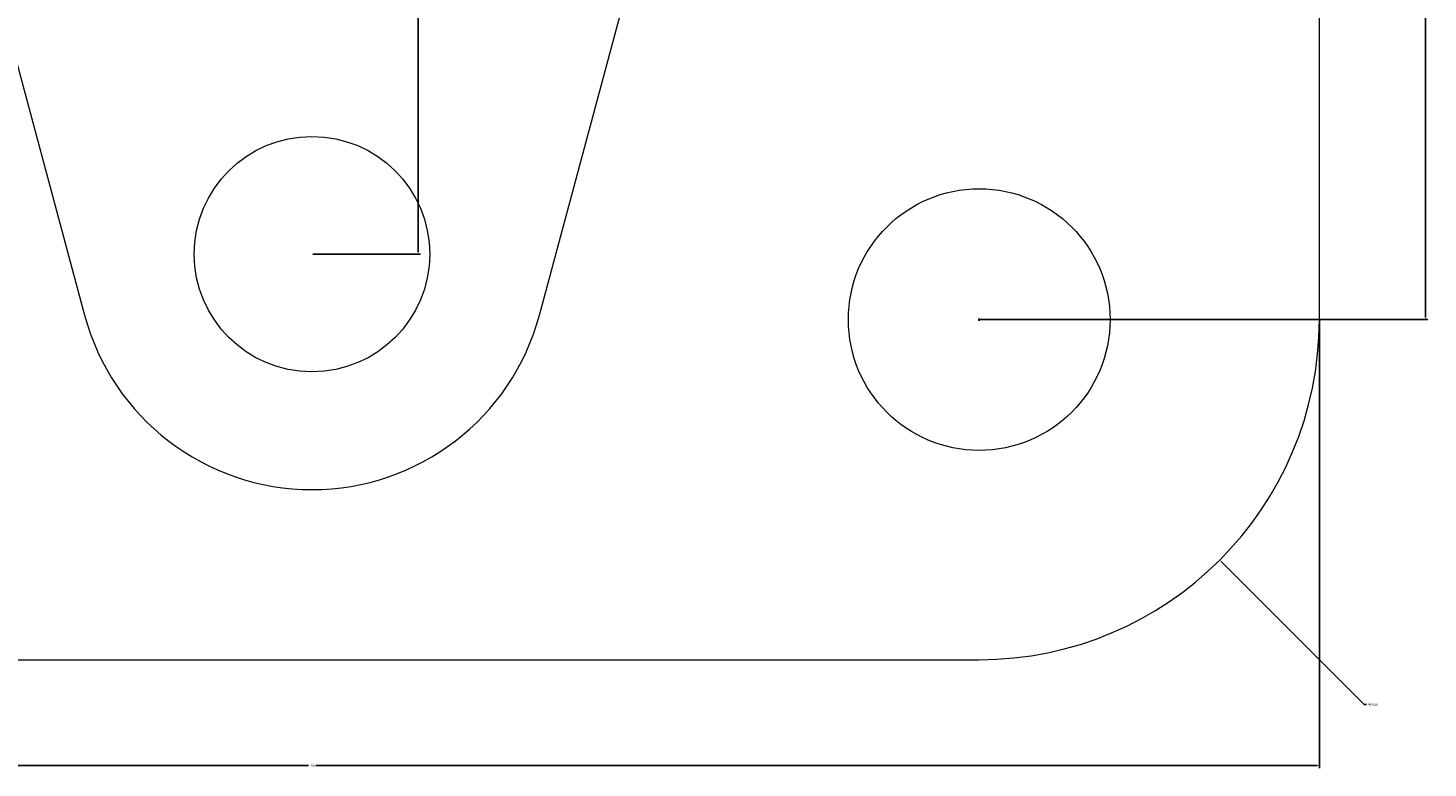
# Model space of a CAD drawing. Units: millimetres. Extents: x 2597 to 2768, y 1809 to 1980.
# Tile 4 of 7: x 2661 to 2768, y 1809 to 1866. Entities that reach past the tile are written whole.
import ezdxf

# ---------------------------------------------------------------- set-up
doc = ezdxf.new("R2010")
doc.units = ezdxf.units.MM
doc.layers.add('M-CONS', color=8, linetype='Continuous', lineweight=18)
doc.layers.add('M-DIMS', color=2, linetype='Continuous', lineweight=18)
doc.styles.get("Standard").update_dxf_attribs({"font": 'arial.ttf'})
doc.dimstyles.get("Standard").update_dxf_attribs({"dimtxt": 0.18, "dimasz": 0.18, "dimexe": 0.18, "dimexo": 0.0625, "dimgap": 0.09, "dimtad": 0, "dimtih": 1, "dimtoh": 1, "dimdec": 4, "dimzin": 0, "dimdsep": 46, "dimtxsty": 'Standard', "dimcen": 0.09, "dimadec": 0, "dimazin": 0, "dimtfac": 1, "dimtdec": 4, "dimtofl": 0, "dimtmove": 0, "dimatfit": 3, "dimfxl": 1, "dimtolj": 1, "dimtzin": 0, "dimarcsym": 0})

# ---------------------------------------------------------------- blocks, each defined once
blk = doc.blocks.new('*D3')
at = {"layer": 'Defpoints', "color": 0, "transparency": 16777216}
for p in [(2605.78, 1843.43), (2759.78, 1843.43), (2759.78, 1809.33)]:
    blk.add_point(p, dxfattribs=at)
at = {"layer": 'M-DIMS', "color": 0, "lineweight": -2, "transparency": 16777216}
for p, q in [((2605.78, 1843.37), (2605.78, 1809.15)), ((2759.78, 1843.37), (2759.78, 1809.15)), ((2605.96, 1809.33), (2682.5, 1809.33)), ((2759.6, 1809.33), (2683.06, 1809.33))]:
    blk.add_line(p, q, dxfattribs=at)
at = {"layer": 'M-DIMS', "color": 0, "transparency": 16777216}
for points in [[(2605.96, 1809.36), (2605.96, 1809.3), (2605.78, 1809.33)], [(2759.6, 1809.36), (2759.6, 1809.3), (2759.78, 1809.33)]]:
    blk.add_solid(points, dxfattribs=at)
at = {"layer": 'M-DIMS', "color": 0, "transparency": 16777216, "insert": (2682.78, 1809.33), "char_height": 0.18, "attachment_point": 5}
blk.add_mtext('\\A1;154', dxfattribs=at)
blk = doc.blocks.new('*D6')
at = {"layer": 'Defpoints', "color": 0, "transparency": 16777216}
for p in [(2733.78, 1945.43), (2767.88, 1945.43), (2733.78, 1843.43)]:
    blk.add_point(p, dxfattribs=at)
at = {"layer": 'M-DIMS', "color": 0, "lineweight": -2, "transparency": 16777216}
for p, q in [((2733.84, 1945.43), (2768.06, 1945.43)), ((2767.88, 1945.25), (2767.88, 1894.61)), ((2767.88, 1843.61), (2767.88, 1894.25)), ((2733.84, 1843.43), (2768.06, 1843.43))]:
    blk.add_line(p, q, dxfattribs=at)
at = {"layer": 'M-DIMS', "color": 0, "transparency": 16777216}
for points in [[(2767.85, 1945.25), (2767.91, 1945.25), (2767.88, 1945.43)], [(2767.85, 1843.61), (2767.91, 1843.61), (2767.88, 1843.43)]]:
    blk.add_solid(points, dxfattribs=at)
at = {"layer": 'M-DIMS', "color": 0, "transparency": 16777216, "insert": (2767.88, 1894.43), "char_height": 0.18, "attachment_point": 5}
blk.add_mtext('\\A1;102', dxfattribs=at)
blk = doc.blocks.new('*D7')
at = {"layer": 'Defpoints', "color": 0, "transparency": 16777216}
for p in [(2682.78, 1894.43), (2682.78, 1848.43), (2690.88, 1848.43)]:
    blk.add_point(p, dxfattribs=at)
at = {"layer": 'M-DIMS', "color": 0, "lineweight": -2, "transparency": 16777216}
for p, q in [((2682.84, 1894.43), (2691.06, 1894.43)), ((2690.88, 1894.25), (2690.88, 1871.61)), ((2690.88, 1848.61), (2690.88, 1871.25)), ((2682.84, 1848.43), (2691.06, 1848.43))]:
    blk.add_line(p, q, dxfattribs=at)
at = {"layer": 'M-DIMS', "color": 0, "transparency": 16777216}
for points in [[(2690.85, 1894.25), (2690.91, 1894.25), (2690.88, 1894.43)], [(2690.85, 1848.61), (2690.91, 1848.61), (2690.88, 1848.43)]]:
    blk.add_solid(points, dxfattribs=at)
at = {"layer": 'M-DIMS', "color": 0, "transparency": 16777216, "insert": (2690.88, 1871.43), "char_height": 0.18, "attachment_point": 5}
blk.add_mtext('\\A1;46', dxfattribs=at)
blk = doc.blocks.new('*D13')
at = {"layer": 'Defpoints', "color": 0, "transparency": 16777216}
for p in [(2733.78, 1843.43), (2752.16, 1825.04)]:
    blk.add_point(p, dxfattribs=at)
at = {"layer": 'M-DIMS', "color": 0, "lineweight": -2, "transparency": 16777216}
for p, q in [((2733.69, 1843.43), (2733.87, 1843.43)), ((2733.78, 1843.34), (2733.78, 1843.52)), ((2763.19, 1814.01), (2752.29, 1824.92)), ((2763.37, 1814.01), (2763.19, 1814.01))]:
    blk.add_line(p, q, dxfattribs=at)
at = {"layer": 'M-DIMS', "color": 0, "transparency": 16777216}
blk.add_solid([(2752.31, 1824.94), (2752.27, 1824.9), (2752.16, 1825.04)], dxfattribs=at)
at = {"layer": 'M-DIMS', "color": 0, "transparency": 16777216, "insert": (2763.87, 1814.01), "char_height": 0.18, "attachment_point": 5}
blk.add_mtext('\\A1;4X R26', dxfattribs=at)

msp = doc.modelspace()

# ---------------------------------------------------------------- linework, layer by layer
at = {"layer": 'M-CONS'}
msp.add_lwpolyline([(2631.7756, 1817.4301), (2733.7756, 1817.4301, 0.41421356), (2759.7756, 1843.4301), (2759.7756, 1945.4301, 0.41421356), (2733.7756, 1971.4301), (2631.7756, 1971.4301, 0.41421356), (2605.7756, 1945.4301), (2605.7756, 1843.4301, 0.41421356)], format="xyb", close=True, dxfattribs=at)
msp.add_lwpolyline([(2713.7756, 1903.4301), (2745.7756, 1903.4301), (2745.7756, 1913.4301), (2708.6698, 1913.4301), (2700.1588, 1945.1014, 0.76675137), (2665.3923, 1945.1014), (2656.8814, 1913.4301), (2619.7756, 1913.4301), (2619.7756, 1903.4301), (2651.7756, 1903.4301), (2651.7756, 1885.4301), (2619.7756, 1885.4301), (2619.7756, 1875.4301), (2656.8814, 1875.4301), (2665.3923, 1843.7587, 0.76675137), (2700.1588, 1843.7587), (2708.6698, 1875.4301), (2745.7756, 1875.4301), (2745.7756, 1885.4301), (2713.7756, 1885.4301), (2713.7756, 1903.4301), (2713.7756, 1894.4301)], format="xyb", dxfattribs=at)
for centre, radius in [((2682.7756, 1848.4301), 9), ((2733.7756, 1843.4301), 10)]:
    msp.add_circle(centre, radius, dxfattribs=at)

# ---------------------------------------------------------------- dimensions: what is measured, and where the dimension line sits
at = {"layer": 'M-DIMS'}
for base, p1, p2, angle, picture, middle in [((2767.8756, 1945.4301), (2733.7756, 1843.4301), (2733.7756, 1945.4301), 90, '*D6', (2767.8756, 1894.4301)), ((2690.8756, 1848.4301), (2682.7756, 1894.4301), (2682.7756, 1848.4301), 270, '*D7', (2690.8756, 1871.4301))]:
    dim = msp.add_linear_dim(base=base, p1=p1, p2=p2, angle=angle, dimstyle='Standard', override={"dimdec": 0, "dimlfac": 1, "dimrnd": 0, "dimzin": 0, "dimdsep": 46, "dimlunit": 2}, dxfattribs=at)
    dim.commit()
    dim.dimension.update_dxf_attribs({"geometry": picture, "text_midpoint": middle})
dim = msp.add_linear_dim(base=(2759.7756, 1809.3301), p1=(2605.7756, 1843.4301), p2=(2759.7756, 1843.4301), dimstyle='Standard', override={"dimdec": 0, "dimlfac": 1, "dimrnd": 0, "dimzin": 0, "dimdsep": 46, "dimlunit": 2}, dxfattribs=at)
dim.commit()
dim.dimension.update_dxf_attribs({"geometry": '*D3', "text_midpoint": (2682.7756, 1809.3301)})
dim = msp.add_radius_dim(center=(2733.7756, 1843.4301), mpoint=(2752.16, 1825.045), text='4X <>', dimstyle='Standard', override={"dimdec": 0, "dimlfac": 1, "dimrnd": 0, "dimzin": 0, "dimdsep": 46, "dimlunit": 2}, dxfattribs=at)
dim.commit()
dim.dimension.update_dxf_attribs({"geometry": '*D13', "text_midpoint": (2763.8727, 1814.0139), "dimtype": 164})

doc.saveas('drawing.dxf')
